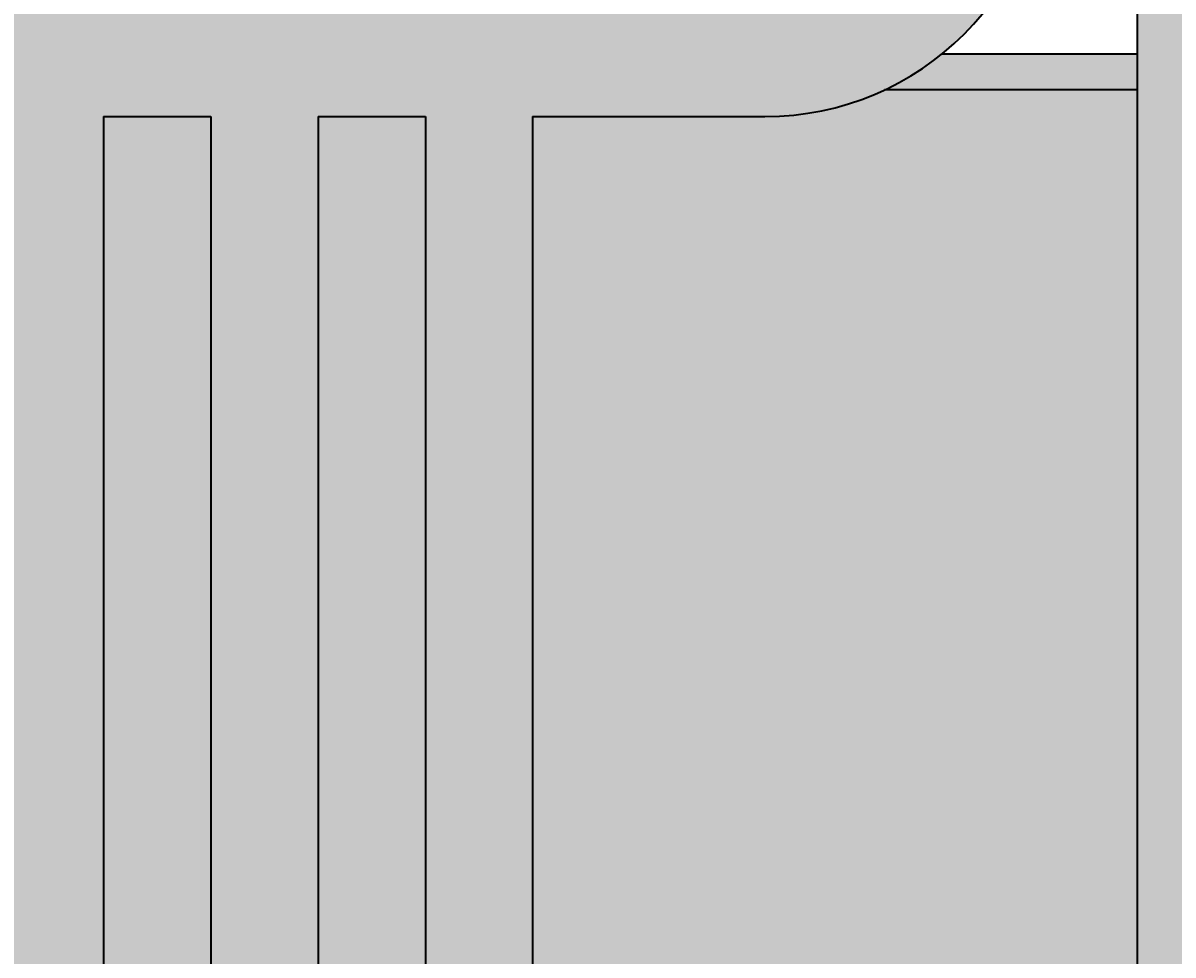
# Model space of a CAD drawing. Units: inches. Extents: x -1 to 292, y -3 to 199.
# Tile 27 of 52: x 148 to 181, y 68 to 95. Entities that reach past the tile are written whole.
import ezdxf

# ---------------------------------------------------------------- set-up
doc = ezdxf.new("R2010")
doc.units = ezdxf.units.IN
doc.header["$MEASUREMENT"] = 0
for name, color, linetype, lineweight in [('M-DIMS', 2, 'Continuous', 18), ('M-EQPM', 7, 'Continuous', 35), ('M-PATT', 8, 'Continuous', 13)]:
    doc.layers.add(name, color=color, linetype=linetype, lineweight=lineweight)
doc.styles.get("Standard").update_dxf_attribs({"font": 'arial.ttf'})
doc.dimstyles.get("Standard").update_dxf_attribs({"dimtxt": 0.18, "dimasz": 0.18, "dimexe": 0.18, "dimexo": 0.0625, "dimgap": 0.09, "dimtad": 0, "dimtih": 1, "dimtoh": 1, "dimdec": 4, "dimzin": 0, "dimdsep": 46, "dimtxsty": 'Standard', "dimcen": 0.09, "dimadec": 0, "dimazin": 0, "dimtfac": 1, "dimtdec": 4, "dimtofl": 0, "dimtmove": 0, "dimatfit": 3, "dimfxl": 1, "dimtolj": 1, "dimtzin": 0, "dimarcsym": 0})

# ---------------------------------------------------------------- blocks, each defined once
blk = doc.blocks.new('BOILER-TUBE')
for p, q in [((0, 40.63), (0, 0)), ((3, 40.63), (3, 0))]:
    blk.add_line(p, q)
for points in [[(0, 40.63), (3, 40.63)], [(3, 0), (0, 0)]]:
    blk.add_lwpolyline(points)
blk = doc.blocks.new('*D10')
at = {"layer": 'Defpoints', "color": 0, "transparency": 16777216}
for p in [(169.176, 99.774), (169.176, 43.391), (292.04, 43.391)]:
    blk.add_point(p, dxfattribs=at)
at = {"layer": 'M-DIMS', "color": 0, "lineweight": -2, "transparency": 16777216}
for p, q in [((169.239, 99.774), (292.22, 99.774)), ((292.04, 99.594), (292.04, 71.764)), ((292.04, 43.571), (292.04, 71.4)), ((169.239, 43.391), (292.22, 43.391))]:
    blk.add_line(p, q, dxfattribs=at)
at = {"layer": 'M-DIMS', "color": 0, "transparency": 16777216}
for points in [[(292.01, 99.594), (292.07, 99.594), (292.04, 99.774)], [(292.01, 43.571), (292.07, 43.571), (292.04, 43.391)]]:
    blk.add_solid(points, dxfattribs=at)
at = {"layer": 'M-DIMS', "color": 0, "transparency": 16777216, "insert": (292.04, 71.582), "char_height": 0.18, "attachment_point": 5}
blk.add_mtext('\\A1;56.38', dxfattribs=at)

msp = doc.modelspace()

# ---------------------------------------------------------------- hatches: boundary and pattern name
at = {"layer": 'M-PATT'}
h = msp.add_hatch(color=256, dxfattribs=at)
h.set_gradient(color1=(0, 127, 0), color2=(0, 127, 0), tint=1, name='CYLINDER')
h.paths.add_polyline_path([(164.5186, 119.2985), (129.9293, 119.2985), (129.9293, 117.2985), (164.1897, 117.2985)])
h.paths.add_polyline_path([(181.5897, 119.2985), (164.5186, 119.2985), (164.1897, 117.2985), (179.5897, 117.2985), (179.5897, 107.8518), (181.5897, 109.1506)])
h.paths.add_polyline_path([(181.5897, 109.1506), (179.5897, 107.8518), (179.5897, 36.2698), (198.4159, 36.2698), (198.4159, 38.2698), (181.5897, 38.2698)])
h.paths.add_polyline_path([(115.4883, 126.765), (111.4883, 126.765), (111.4883, 114.6589), (115.4883, 114.6589)])
h.paths.add_polyline_path([(123.408, 119.2985), (115.4883, 119.2985), (115.4883, 117.2985), (123.408, 117.2985)])
h.paths.add_polyline_path([(115.4883, 112.6589), (111.4883, 112.6589), (111.4883, 106.9941), (115.4883, 106.9941)])
h.paths.add_polyline_path([(120.9032, 106.9941), (106.0735, 106.9941), (106.0735, 105.9941), (120.9032, 105.9941)])
h.paths.add_polyline_path([(236.4209, 117.5104), (234.9209, 117.5104), (234.9209, 97.1861), (236.4209, 97.1861)])
h.paths.add_polyline_path([(236.4209, 126.4904), (234.9209, 126.4904), (234.9209, 118.9331), (236.4209, 118.9331)])
h.paths.add_polyline_path([(244.9552, 125.7269), (242.9552, 125.7269), (242.9552, 116.8562), (244.9552, 116.8562)])
h.paths.add_polyline_path([(244.9552, 115.1721), (242.9552, 115.1721), (242.9552, 109.7385), (244.9552, 109.7385)])
h.paths.add_polyline_path([(248.4468, 109.7385), (239.4637, 109.7385), (239.4637, 109.4289), (248.4468, 109.4289)])
h = msp.add_hatch(color=256, dxfattribs=at)
h.set_gradient(color1=(237, 31, 36), color2=(242, 113, 114), tint=1, name='CYLINDER')
h.paths.add_polyline_path([(106.0735, 105.9941), (106.0735, 106.9941), (108.0603, 106.9941), (107.8488, 107.6501), (57.8007, 107.6501, 0.4142136), (49.9241, 99.7735), (52.3176, 101.3278), (55.0097, 99.7735), (57.4032, 101.3278), (60.0953, 99.7735), (62.4888, 101.3278), (65.1809, 99.7735), (67.5744, 101.3278), (70.2665, 99.7735), (72.66, 101.3278), (75.3521, 99.7735), (77.7456, 101.3278), (80.4377, 99.7735), (82.8312, 101.3278), (85.5233, 99.7735), (87.9168, 101.3278), (90.6089, 99.7735), (93.0024, 101.3278), (95.6945, 99.7735), (98.088, 101.3278), (100.7801, 99.7735), (103.1736, 101.3278), (105.8657, 99.7735), (108.2592, 101.3278), (110.9513, 99.7735), (113.3448, 101.3278), (116.0369, 99.7735), (118.4304, 101.3278), (121.1225, 99.7735), (123.516, 101.3278), (126.2082, 99.7735), (128.6016, 101.3278), (131.2938, 99.7735), (133.6872, 101.3278), (136.3794, 99.7735), (138.7728, 101.3278), (141.465, 99.7735), (143.8584, 101.3278), (146.5506, 99.7735), (148.944, 101.3278), (151.6362, 99.7735), (154.0296, 101.3278), (156.7218, 99.7735), (159.1152, 101.3278), (160.6222, 100.4578), (160.6222, 107.6501), (115.4883, 107.6501), (115.4883, 106.9941), (120.9032, 106.9941), (120.9032, 105.9941), (120.9032, 103.3981), (106.0735, 103.3981)])
h.paths.add_polyline_path([(169.176, 107.6501), (162.1623, 107.6501), (162.1623, 100.004), (164.2008, 101.3278), (166.893, 99.7735), (169.2864, 101.3278), (171.9786, 99.7735), (174.372, 101.3278), (177.0526, 99.7802, 0.4139642)])
h.paths.add_polyline_path([(111.4883, 107.6501), (107.8488, 107.6501), (108.0603, 106.9941), (111.4883, 106.9941)], flags=17)
h.paths.add_polyline_path([(61.6788, 91.897), (57.8007, 91.897, -0.1099266), (54.4604, 92.6403), (43.2011, 92.6403), (23.9502, 84.4688), (23.9502, 58.376), (43.2011, 47.2615), (50.9409, 47.2615, -0.2705926), (57.8007, 51.2672), (61.6788, 51.2672)])
h.paths.add_polyline_path([(73.6788, 91.897), (70.6788, 91.897), (70.6788, 51.2672), (73.6788, 51.2672)])
h.paths.add_polyline_path([(79.6788, 91.897), (76.6788, 91.897), (76.6788, 51.2672), (79.6788, 51.2672)])
h.paths.add_polyline_path([(67.6788, 91.897), (64.6788, 91.897), (64.6788, 51.2672), (67.6788, 51.2672)])
h.paths.add_polyline_path([(101.6788, 91.897), (82.6788, 91.897), (82.6788, 51.2672), (101.6788, 51.2672)])
h.paths.add_polyline_path([(107.6788, 91.897), (104.6788, 91.897), (104.6788, 51.2672), (107.6788, 51.2672)])
h.paths.add_polyline_path([(113.6788, 91.897), (110.6788, 91.897), (110.6788, 51.2672), (113.6788, 51.2672)])
h.paths.add_polyline_path([(119.6788, 91.897), (116.6788, 91.897), (116.6788, 51.2672), (119.6788, 51.2672)])
h.paths.add_polyline_path([(141.6788, 91.897), (122.6788, 91.897), (122.6788, 51.2672), (141.6788, 51.2672)])
h.paths.add_polyline_path([(147.6788, 91.897), (144.6788, 91.897), (144.6788, 51.2672), (147.6788, 51.2672)])
h.paths.add_polyline_path([(153.6788, 91.897), (150.6788, 91.897), (150.6788, 51.2672), (153.6788, 51.2672)])
h.paths.add_polyline_path([(159.6788, 91.897), (156.6788, 91.897), (156.6788, 51.2672), (159.6788, 51.2672)])
h.paths.add_polyline_path([(179.5897, 92.6403), (172.5163, 92.6403, -0.1099266), (169.176, 91.897), (162.6788, 91.897), (162.6788, 51.2672), (169.176, 51.2672, -0.2705926), (176.0358, 47.2615), (179.5897, 47.2615)])
h.paths.add_polyline_path([(203.0265, 84.4688), (183.7755, 92.6403), (181.5897, 92.6403), (181.5897, 47.2615), (183.7755, 47.2615), (203.0265, 58.376)])
h.paths.add_polyline_path([(184.4188, 61.52), (200.7224, 61.52), (200.7224, 77.7532), (184.4188, 77.7532)], flags=24)
h = msp.add_hatch(color=256, dxfattribs=at)
h.set_gradient(color1=(0, 255, 255), color2=(0, 255, 255), tint=1)
h.paths.add_polyline_path([(75.3521, 99.7735), (72.66, 101.3278), (70.2665, 99.7735), (67.5744, 101.3278), (65.1809, 99.7735), (62.4888, 101.3278), (60.0953, 99.7735), (57.4032, 101.3278), (55.0097, 99.7735), (52.3176, 101.3278), (49.9241, 99.7735, 0.4142136), (57.8007, 91.897), (61.6788, 91.897), (61.6788, 51.2672), (57.8007, 51.2672, 0.8088808), (54.5813, 36.2021), (65.0947, 51.2672), (64.6788, 51.2672), (64.6788, 91.897), (67.6788, 91.897), (67.6788, 51.2672), (65.0947, 51.2672), (54.5813, 36.2021, 0.1056561), (57.8007, 35.5141), (169.176, 35.5141, 1), (169.176, 51.2672), (162.6788, 51.2672), (162.6788, 91.897), (169.176, 91.897, 0.4144629), (177.0526, 99.7802), (174.372, 101.3278), (171.9786, 99.7735), (169.2864, 101.3278), (166.893, 99.7735), (164.2008, 101.3278), (162.1623, 100.004), (162.1623, 96.1027), (160.6222, 96.1027), (160.6222, 100.4578), (159.1152, 101.3278), (156.7218, 99.7735), (154.0296, 101.3278), (151.6362, 99.7735), (148.944, 101.3278), (146.5506, 99.7735), (143.8584, 101.3278), (141.465, 99.7735), (138.7728, 101.3278), (136.3794, 99.7735), (133.6872, 101.3278), (131.2938, 99.7735), (128.6016, 101.3278), (126.2082, 99.7735), (123.516, 101.3278), (121.1225, 99.7735), (118.4304, 101.3278), (116.0369, 99.7735), (113.3448, 101.3278), (110.9513, 99.7735), (108.2592, 101.3278), (105.8657, 99.7735), (103.1736, 101.3278), (100.7801, 99.7735), (98.088, 101.3278), (95.6945, 99.7735), (93.0024, 101.3278), (90.6089, 99.7735), (87.9168, 101.3278), (85.5233, 99.7735), (82.8312, 101.3278), (80.4377, 99.7735), (77.7456, 101.3278)])
h.paths.add_polyline_path([(79.6788, 91.897), (79.6788, 51.2672), (76.6788, 51.2672), (76.6788, 91.897)], flags=16)
h.paths.add_polyline_path([(73.6788, 91.897), (73.6788, 51.2672), (70.6788, 51.2672), (70.6788, 91.897)], flags=16)
h.paths.add_polyline_path([(82.6788, 91.897), (101.6788, 91.897), (101.6788, 51.2672), (82.6788, 51.2672)], flags=16)
h.paths.add_polyline_path([(104.6788, 91.897), (107.6788, 91.897), (107.6788, 51.2672), (104.6788, 51.2672)], flags=16)
h.paths.add_polyline_path([(110.6788, 91.897), (113.6788, 91.897), (113.6788, 51.2672), (110.6788, 51.2672)], flags=16)
h.paths.add_polyline_path([(116.6788, 91.897), (119.6788, 91.897), (119.6788, 51.2672), (116.6788, 51.2672)], flags=16)
h.paths.add_polyline_path([(122.6788, 91.897), (141.6788, 91.897), (141.6788, 51.2672), (144.6788, 51.2672), (144.6788, 91.897), (147.6788, 91.897), (147.6788, 51.2672), (122.6788, 51.2672)], flags=16)
h.paths.add_polyline_path([(150.6788, 91.897), (153.6788, 91.897), (153.6788, 51.2672), (150.6788, 51.2672)], flags=16)
h.paths.add_polyline_path([(156.6788, 91.897), (159.6788, 91.897), (159.6788, 51.2672), (156.6788, 51.2672)], flags=16)
h = msp.add_hatch(color=256, dxfattribs=at)
h.set_gradient(color1=(76, 38, 47), color2=(76, 38, 47), tint=1, name='CYLINDER')
h.paths.add_polyline_path([(40.8628, 91.6478), (40.3591, 92.5203), (23.9502, 85.5552), (23.9502, 84.4688)])
h.paths.add_polyline_path([(52.8586, 93.6403), (42.9977, 93.6403), (40.3591, 92.5203), (40.8628, 91.6478), (43.2011, 92.6403), (54.4604, 92.6403, -0.0601508)])
h.paths.add_polyline_path([(23.9502, 88.5821), (21.8612, 88.5821), (21.8612, 54.5821), (23.9502, 54.5821)])
h.paths.add_polyline_path([(23.9502, 58.376), (23.9502, 57.2213), (42.9332, 46.2615), (50.4659, 46.2615, -0.0351813), (50.9409, 47.2615), (43.2011, 47.2615)])
h.paths.add_polyline_path([(179.5897, 93.6403), (174.1181, 93.6403, -0.0601508), (172.5163, 92.6403), (179.5897, 92.6403)])
h.paths.add_polyline_path([(183.979, 93.6403), (181.5897, 93.6403), (181.5897, 92.6403), (183.7755, 92.6403), (203.0265, 84.4688), (203.0265, 85.5552)])
h.paths.add_polyline_path([(205.1155, 88.5821), (203.0265, 88.5821), (203.0265, 54.5821), (205.1155, 54.5821)])
h.paths.add_polyline_path([(203.0265, 57.2213), (203.0265, 58.376), (183.7755, 47.2615), (181.5897, 47.2615), (181.5897, 46.2615), (184.0435, 46.2615)])
h.paths.add_polyline_path([(179.5897, 47.2615), (176.0358, 47.2615, -0.0351813), (176.5107, 46.2615), (179.5897, 46.2615)])

# ---------------------------------------------------------------- linework, layer by layer
at = {"layer": 'M-EQPM'}
msp.add_line((162.6788, 91.897), (162.6788, 51.2672), dxfattribs=at)
for points in [[(129.9293, 117.2985), (179.5897, 117.2985), (179.5897, 36.2698)], [(179.5897, 93.6403), (174.1181, 93.6403)], [(179.5897, 92.6403), (172.5163, 92.6403)]]:
    msp.add_lwpolyline(points, dxfattribs=at)
msp.add_lwpolyline([(162.6788, 91.897), (169.176, 91.897, 1), (169.176, 107.6501), (162.1623, 107.6501)], format="xyb", dxfattribs=at)

# ---------------------------------------------------------------- block references
for p in [(150.679, 51.267), (156.679, 51.267)]:
    msp.add_blockref('BOILER-TUBE', p, dxfattribs=at)

# ---------------------------------------------------------------- dimensions: what is measured, and where the dimension line sits
at = {"layer": 'M-DIMS'}
dim = msp.add_linear_dim(base=(292.0399, 43.3906), p1=(169.176, 99.7735), p2=(169.176, 43.3906), angle=90, dimstyle='Standard', override={"dimdec": 2, "dimlfac": 1, "dimrnd": 0, "dimzin": 0, "dimdsep": 46, "dimlunit": 2}, dxfattribs=at)
dim.commit()
dim.dimension.update_dxf_attribs({"geometry": '*D10', "text_midpoint": (292.0399, 71.5821)})

doc.saveas('drawing.dxf')
